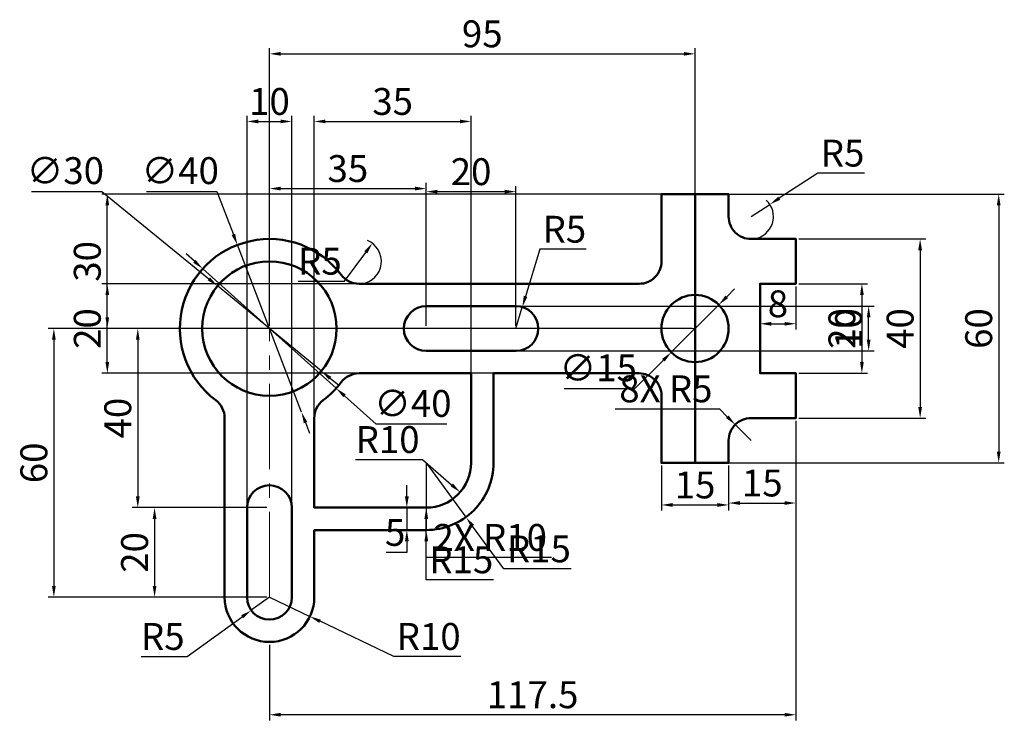
# Model space of a CAD drawing. Units: millimetres. Extents: x 35 to 255, y -2 to 154.
import ezdxf

# ---------------------------------------------------------------- set-up
doc = ezdxf.new("R2010")
doc.units = ezdxf.units.MM
doc.linetypes.add('CENTER2', pattern=[28.575, 19.05, -3.175, 3.175, -3.175])
for name, color, linetype, lineweight in [('M-CNTR', 4, 'CENTER2', 18), ('M-DIMS', 2, 'Continuous', 25), ('M-OUTL', 7, 'Continuous', 50)]:
    doc.layers.add(name, color=color, linetype=linetype, lineweight=lineweight)
doc.styles.get("Standard").update_dxf_attribs({"font": 'arial.ttf'})
doc.dimstyles.new('ISO-25', dxfattribs={"dimtxt": 6, "dimasz": 2.5, "dimexe": 1.25, "dimexo": 0.625, "dimtad": 1, "dimtoh": 1, "dimdec": 0, "dimtxsty": 'Standard', "dimcen": 2.5, "dimadec": 0, "dimazin": 0, "dimtfac": 1, "dimtdec": 0, "dimtmove": 0, "dimatfit": 3, "dimfxl": 1, "dimarcsym": 0})

# ---------------------------------------------------------------- blocks, each defined once
blk = doc.blocks.new('*D1')
at = {"layer": 'Defpoints', "color": 0, "transparency": 16777216}
for p in [(186.1, 146.8), (91.1, 85.45), (186.1, 85.45)]:
    blk.add_point(p, dxfattribs=at)
at = {"layer": 'M-DIMS', "color": 0, "lineweight": -2, "transparency": 16777216}
for p, q in [((91.1, 86.08), (91.1, 148.05)), ((186.1, 86.08), (186.1, 148.05)), ((93.6, 146.8), (183.6, 146.8))]:
    blk.add_line(p, q, dxfattribs=at)
at = {"layer": 'M-DIMS', "color": 0, "transparency": 16777216}
for points in [[(93.6, 147.22), (93.6, 146.39), (91.1, 146.8)], [(183.6, 147.22), (183.6, 146.39), (186.1, 146.8)]]:
    blk.add_solid(points, dxfattribs=at)
at = {"layer": 'M-DIMS', "color": 0, "transparency": 16777216, "insert": (138.6, 150.49), "char_height": 6, "attachment_point": 5}
blk.add_mtext('95', dxfattribs=at)
blk = doc.blocks.new('*D2')
at = {"layer": 'Defpoints', "color": 0, "transparency": 16777216}
for p in [(126.1, 116.71), (91.1, 85.45), (126.1, 85.45)]:
    blk.add_point(p, dxfattribs=at)
at = {"layer": 'M-DIMS', "color": 0, "lineweight": -2, "transparency": 16777216}
for p, q in [((91.1, 86.08), (91.1, 117.96)), ((93.6, 116.71), (123.6, 116.71)), ((126.1, 86.08), (126.1, 117.96))]:
    blk.add_line(p, q, dxfattribs=at)
at = {"layer": 'M-DIMS', "color": 0, "transparency": 16777216}
for points in [[(93.6, 117.13), (93.6, 116.3), (91.1, 116.71)], [(123.6, 117.13), (123.6, 116.3), (126.1, 116.71)]]:
    blk.add_solid(points, dxfattribs=at)
at = {"layer": 'M-DIMS', "color": 0, "transparency": 16777216, "insert": (108.6, 120.4), "char_height": 6, "attachment_point": 5}
blk.add_mtext('35', dxfattribs=at)
blk = doc.blocks.new('*D3')
at = {"layer": 'Defpoints', "color": 0, "transparency": 16777216}
for p in [(146.1, 116.02), (126.1, 85.45), (146.1, 85.45)]:
    blk.add_point(p, dxfattribs=at)
at = {"layer": 'M-DIMS', "color": 0, "lineweight": -2, "transparency": 16777216}
for p, q in [((126.1, 86.08), (126.1, 117.27)), ((146.1, 86.08), (146.1, 117.27)), ((128.6, 116.02), (143.6, 116.02))]:
    blk.add_line(p, q, dxfattribs=at)
at = {"layer": 'M-DIMS', "color": 0, "transparency": 16777216}
for points in [[(128.6, 116.44), (128.6, 115.61), (126.1, 116.02)], [(143.6, 116.44), (143.6, 115.61), (146.1, 116.02)]]:
    blk.add_solid(points, dxfattribs=at)
at = {"layer": 'M-DIMS', "color": 0, "transparency": 16777216, "insert": (136.1, 119.71), "char_height": 6, "attachment_point": 5}
blk.add_mtext('20', dxfattribs=at)
blk = doc.blocks.new('*D4')
at = {"layer": 'Defpoints', "color": 0, "transparency": 16777216}
for p in [(202.79, 113.18), (198.6, 110.45)]:
    blk.add_point(p, dxfattribs=at)
at = {"layer": 'M-DIMS', "color": 0, "lineweight": -2, "transparency": 16777216}
for p, q in [((213.54, 120.17), (204.89, 114.54)), ((223.89, 120.17), (213.54, 120.17)), ((198.6, 110.45), (202.79, 113.18))]:
    blk.add_line(p, q, dxfattribs=at)
blk.add_arc((198.6, 110.45), 5, 277.162, 47.3684, dxfattribs=at)
at = {"layer": 'M-DIMS', "color": 0, "transparency": 16777216}
blk.add_solid([(204.66, 114.89), (205.12, 114.19), (202.79, 113.18)], dxfattribs=at)
at = {"layer": 'M-DIMS', "color": 0, "transparency": 16777216, "insert": (219.03, 123.85), "char_height": 6, "attachment_point": 5}
blk.add_mtext('R5', dxfattribs=at)
blk = doc.blocks.new('*D5')
at = {"layer": 'Defpoints', "color": 0, "transparency": 16777216}
for p in [(200.6, 95.45), (208.6, 95.45), (208.6, 86.52)]:
    blk.add_point(p, dxfattribs=at)
at = {"layer": 'M-DIMS', "color": 0, "lineweight": -2, "transparency": 16777216}
for p, q in [((200.6, 94.83), (200.6, 85.27)), ((208.6, 94.83), (208.6, 85.27)), ((203.1, 86.52), (206.1, 86.52))]:
    blk.add_line(p, q, dxfattribs=at)
at = {"layer": 'M-DIMS', "color": 0, "transparency": 16777216}
for points in [[(203.1, 86.93), (203.1, 86.1), (200.6, 86.52)], [(206.1, 86.93), (206.1, 86.1), (208.6, 86.52)]]:
    blk.add_solid(points, dxfattribs=at)
at = {"layer": 'M-DIMS', "color": 0, "transparency": 16777216, "insert": (204.6, 90.2), "char_height": 6, "attachment_point": 5}
blk.add_mtext('8', dxfattribs=at)
blk = doc.blocks.new('*D6')
at = {"layer": 'Defpoints', "color": 0, "transparency": 16777216}
for p in [(208.6, 95.45), (208.6, 75.45), (223.34, 75.45)]:
    blk.add_point(p, dxfattribs=at)
at = {"layer": 'M-DIMS', "color": 0, "lineweight": -2, "transparency": 16777216}
for p, q in [((209.23, 95.45), (224.59, 95.45)), ((223.34, 92.95), (223.34, 77.95)), ((209.23, 75.45), (224.59, 75.45))]:
    blk.add_line(p, q, dxfattribs=at)
at = {"layer": 'M-DIMS', "color": 0, "transparency": 16777216}
for points in [[(222.93, 92.95), (223.76, 92.95), (223.34, 95.45)], [(222.93, 77.95), (223.76, 77.95), (223.34, 75.45)]]:
    blk.add_solid(points, dxfattribs=at)
at = {"layer": 'M-DIMS', "color": 0, "transparency": 16777216, "insert": (219.66, 85.45), "char_height": 6, "attachment_point": 5, "rotation": 90}
blk.add_mtext('20', dxfattribs=at)
blk = doc.blocks.new('*D7')
at = {"layer": 'Defpoints', "color": 0, "transparency": 16777216}
for p in [(208.6, 105.45), (208.6, 65.45), (236.34, 65.45)]:
    blk.add_point(p, dxfattribs=at)
at = {"layer": 'M-DIMS', "color": 0, "lineweight": -2, "transparency": 16777216}
for p, q in [((209.23, 105.45), (237.59, 105.45)), ((236.34, 102.95), (236.34, 67.95)), ((209.23, 65.45), (237.59, 65.45))]:
    blk.add_line(p, q, dxfattribs=at)
at = {"layer": 'M-DIMS', "color": 0, "transparency": 16777216}
for points in [[(235.92, 102.95), (236.76, 102.95), (236.34, 105.45)], [(235.92, 67.95), (236.76, 67.95), (236.34, 65.45)]]:
    blk.add_solid(points, dxfattribs=at)
at = {"layer": 'M-DIMS', "color": 0, "transparency": 16777216, "insert": (232.65, 85.45), "char_height": 6, "attachment_point": 5, "rotation": 90}
blk.add_mtext('40', dxfattribs=at)
blk = doc.blocks.new('*D8')
at = {"layer": 'Defpoints', "color": 0, "transparency": 16777216}
for p in [(178.6, 55.45), (193.6, 55.45), (193.6, 46.05)]:
    blk.add_point(p, dxfattribs=at)
at = {"layer": 'M-DIMS', "color": 0, "lineweight": -2, "transparency": 16777216}
for p, q in [((178.6, 54.83), (178.6, 44.8)), ((193.6, 54.83), (193.6, 44.8)), ((181.1, 46.05), (191.1, 46.05))]:
    blk.add_line(p, q, dxfattribs=at)
at = {"layer": 'M-DIMS', "color": 0, "transparency": 16777216}
for points in [[(181.1, 46.47), (181.1, 45.63), (178.6, 46.05)], [(191.1, 46.47), (191.1, 45.63), (193.6, 46.05)]]:
    blk.add_solid(points, dxfattribs=at)
at = {"layer": 'M-DIMS', "color": 0, "transparency": 16777216, "insert": (186.1, 49.74), "char_height": 6, "attachment_point": 5}
blk.add_mtext('15', dxfattribs=at)
blk = doc.blocks.new('*D9')
at = {"layer": 'Defpoints', "color": 0, "transparency": 16777216}
for p in [(208.6, 65.45), (193.6, 55.45), (208.6, 46.48)]:
    blk.add_point(p, dxfattribs=at)
at = {"layer": 'M-DIMS', "color": 0, "lineweight": -2, "transparency": 16777216}
for p, q in [((208.6, 64.83), (208.6, 45.23)), ((193.6, 54.83), (193.6, 45.23)), ((196.1, 46.48), (206.1, 46.48))]:
    blk.add_line(p, q, dxfattribs=at)
at = {"layer": 'M-DIMS', "color": 0, "transparency": 16777216}
for points in [[(196.1, 46.9), (196.1, 46.07), (193.6, 46.48)], [(206.1, 46.9), (206.1, 46.07), (208.6, 46.48)]]:
    blk.add_solid(points, dxfattribs=at)
at = {"layer": 'M-DIMS', "color": 0, "transparency": 16777216, "insert": (201.1, 50.17), "char_height": 6, "attachment_point": 5}
blk.add_mtext('15', dxfattribs=at)
blk = doc.blocks.new('*D10')
at = {"layer": 'Defpoints', "color": 0, "transparency": 16777216}
for p in [(186.1, 115.45), (186.1, 55.45), (253.88, 55.45)]:
    blk.add_point(p, dxfattribs=at)
at = {"layer": 'M-DIMS', "color": 0, "lineweight": -2, "transparency": 16777216}
for p, q in [((186.73, 115.45), (255.13, 115.45)), ((253.88, 112.95), (253.88, 57.95)), ((186.73, 55.45), (255.13, 55.45))]:
    blk.add_line(p, q, dxfattribs=at)
at = {"layer": 'M-DIMS', "color": 0, "transparency": 16777216}
for points in [[(253.46, 112.95), (254.3, 112.95), (253.88, 115.45)], [(253.46, 57.95), (254.3, 57.95), (253.88, 55.45)]]:
    blk.add_solid(points, dxfattribs=at)
at = {"layer": 'M-DIMS', "color": 0, "transparency": 16777216, "insert": (250.19, 85.45), "char_height": 6, "attachment_point": 5, "rotation": 90}
blk.add_mtext('60', dxfattribs=at)
blk = doc.blocks.new('*D11')
at = {"layer": 'Defpoints', "color": 0, "transparency": 16777216}
for p in [(147.54, 90.24), (146.1, 85.45)]:
    blk.add_point(p, dxfattribs=at)
at = {"layer": 'M-DIMS', "color": 0, "lineweight": -2, "transparency": 16777216}
for p, q in [((151.44, 103.18), (148.27, 92.64)), ((161.79, 103.18), (151.44, 103.18)), ((146.1, 85.45), (147.54, 90.24))]:
    blk.add_line(p, q, dxfattribs=at)
at = {"layer": 'M-DIMS', "color": 0, "transparency": 16777216}
blk.add_solid([(147.87, 92.76), (148.66, 92.51), (147.54, 90.24)], dxfattribs=at)
at = {"layer": 'M-DIMS', "color": 0, "transparency": 16777216, "insert": (156.93, 106.85), "char_height": 6, "attachment_point": 5}
blk.add_mtext('R5', dxfattribs=at)
blk = doc.blocks.new('*D12')
at = {"layer": 'Defpoints', "color": 0, "transparency": 16777216}
for p in [(114.07, 104.48), (111.1, 100.45)]:
    blk.add_point(p, dxfattribs=at)
at = {"layer": 'M-DIMS', "color": 0, "lineweight": -2, "transparency": 16777216}
for p, q in [((107.85, 96.04), (112.58, 102.47)), ((97.5, 96.04), (107.85, 96.04))]:
    blk.add_line(p, q, dxfattribs=at)
blk.add_arc((111.1, 100.45), 5, 277.162, 67.9535, dxfattribs=at)
at = {"layer": 'M-DIMS', "color": 0, "transparency": 16777216}
blk.add_solid([(112.25, 102.71), (112.92, 102.22), (114.07, 104.48)], dxfattribs=at)
at = {"layer": 'M-DIMS', "color": 0, "transparency": 16777216, "insert": (102.36, 99.71), "char_height": 6, "attachment_point": 5}
blk.add_mtext('R5', dxfattribs=at)
blk = doc.blocks.new('*D13')
at = {"layer": 'Defpoints', "color": 0, "transparency": 16777216}
for p in [(126.1, 55.45), (133.66, 48.91)]:
    blk.add_point(p, dxfattribs=at)
at = {"layer": 'M-DIMS', "color": 0, "lineweight": -2, "transparency": 16777216}
for p, q in [((110.31, 56.19), (125.25, 56.19)), ((125.25, 56.19), (131.77, 50.55))]:
    blk.add_line(p, q, dxfattribs=at)
at = {"layer": 'M-DIMS', "color": 0, "transparency": 16777216}
blk.add_solid([(132.05, 50.86), (131.5, 50.23), (133.66, 48.91)], dxfattribs=at)
at = {"layer": 'M-DIMS', "color": 0, "transparency": 16777216, "insert": (117.47, 59.88), "char_height": 6, "attachment_point": 5}
blk.add_mtext('R10', dxfattribs=at)
blk = doc.blocks.new('*D14')
at = {"layer": 'Defpoints', "color": 0, "transparency": 16777216}
for p in [(126.1, 55.45), (134.96, 43.35)]:
    blk.add_point(p, dxfattribs=at)
at = {"layer": 'M-DIMS', "color": 0, "lineweight": -2, "transparency": 16777216}
for p, q in [((126.1, 55.45), (134.96, 43.35)), ((143.43, 31.77), (136.43, 41.33)), ((158.44, 31.77), (143.43, 31.77))]:
    blk.add_line(p, q, dxfattribs=at)
at = {"layer": 'M-DIMS', "color": 0, "transparency": 16777216}
blk.add_solid([(136.77, 41.58), (136.1, 41.08), (134.96, 43.35)], dxfattribs=at)
at = {"layer": 'M-DIMS', "color": 0, "transparency": 16777216, "insert": (151.24, 35.46), "char_height": 6, "attachment_point": 5}
blk.add_mtext('R15', dxfattribs=at)
blk = doc.blocks.new('*D15')
at = {"layer": 'Defpoints', "color": 0, "transparency": 16777216}
for p in [(119.82, 45.45), (119.82, 40.45), (121.77, 40.45)]:
    blk.add_point(p, dxfattribs=at)
at = {"layer": 'M-DIMS', "color": 0, "lineweight": -2, "transparency": 16777216}
for p, q in [((121.77, 47.95), (121.77, 50.45)), ((120.45, 45.45), (123.02, 45.45)), ((121.77, 45.45), (121.77, 40.45)), ((120.45, 40.45), (123.02, 40.45)), ((121.77, 37.95), (121.77, 35.45)), ((121.77, 35.45), (117.17, 35.45))]:
    blk.add_line(p, q, dxfattribs=at)
at = {"layer": 'M-DIMS', "color": 0, "transparency": 16777216}
for points in [[(121.35, 47.95), (122.19, 47.95), (121.77, 45.45)], [(121.35, 37.95), (122.19, 37.95), (121.77, 40.45)]]:
    blk.add_solid(points, dxfattribs=at)
at = {"layer": 'M-DIMS', "color": 0, "transparency": 16777216, "insert": (119.16, 39.13), "char_height": 6, "attachment_point": 5}
blk.add_mtext('5', dxfattribs=at)
blk = doc.blocks.new('*D16')
at = {"layer": 'Defpoints', "color": 0, "transparency": 16777216}
for p in [(91.1, 45.45), (65.46, 25.45), (91.1, 25.45)]:
    blk.add_point(p, dxfattribs=at)
at = {"layer": 'M-DIMS', "color": 0, "lineweight": -2, "transparency": 16777216}
for p, q in [((90.48, 45.45), (64.21, 45.45)), ((65.46, 42.95), (65.46, 27.95)), ((90.48, 25.45), (64.21, 25.45))]:
    blk.add_line(p, q, dxfattribs=at)
at = {"layer": 'M-DIMS', "color": 0, "transparency": 16777216}
for points in [[(65.04, 42.95), (65.87, 42.95), (65.46, 45.45)], [(65.04, 27.95), (65.87, 27.95), (65.46, 25.45)]]:
    blk.add_solid(points, dxfattribs=at)
at = {"layer": 'M-DIMS', "color": 0, "transparency": 16777216, "insert": (61.77, 35.45), "char_height": 6, "attachment_point": 5, "rotation": 90}
blk.add_mtext('20', dxfattribs=at)
blk = doc.blocks.new('*D17')
at = {"layer": 'Defpoints', "color": 0, "transparency": 16777216}
for p in [(91.1, 85.45), (61.71, 45.45), (91.1, 45.45)]:
    blk.add_point(p, dxfattribs=at)
at = {"layer": 'M-DIMS', "color": 0, "lineweight": -2, "transparency": 16777216}
for p, q in [((90.48, 85.45), (60.46, 85.45)), ((61.71, 82.95), (61.71, 47.95)), ((90.48, 45.45), (60.46, 45.45))]:
    blk.add_line(p, q, dxfattribs=at)
at = {"layer": 'M-DIMS', "color": 0, "transparency": 16777216}
for points in [[(61.29, 82.95), (62.12, 82.95), (61.71, 85.45)], [(61.29, 47.95), (62.12, 47.95), (61.71, 45.45)]]:
    blk.add_solid(points, dxfattribs=at)
at = {"layer": 'M-DIMS', "color": 0, "transparency": 16777216, "insert": (58.02, 65.45), "char_height": 6, "attachment_point": 5, "rotation": 90}
blk.add_mtext('40', dxfattribs=at)
blk = doc.blocks.new('*D18')
at = {"layer": 'Defpoints', "color": 0, "transparency": 16777216}
for p in [(79.5, 94.96), (102.7, 75.95)]:
    blk.add_point(p, dxfattribs=at)
at = {"layer": 'M-DIMS', "color": 0, "lineweight": -2, "transparency": 16777216}
for p, q in [((37.99, 116.09), (53.72, 116.09)), ((53.72, 116.09), (77.57, 96.55)), ((102.7, 75.95), (79.5, 94.96)), ((104.64, 74.36), (106.57, 72.78))]:
    blk.add_line(p, q, dxfattribs=at)
at = {"layer": 'M-DIMS', "color": 0, "transparency": 16777216}
for points in [[(77.83, 96.87), (77.3, 96.22), (79.5, 94.96)], [(104.9, 74.68), (104.37, 74.04), (102.7, 75.95)]]:
    blk.add_solid(points, dxfattribs=at)
at = {"layer": 'M-DIMS', "color": 0, "transparency": 16777216, "insert": (45.54, 119.94), "char_height": 6, "attachment_point": 5}
blk.add_mtext('∅30', dxfattribs=at)
blk = doc.blocks.new('*D19')
at = {"layer": 'Defpoints', "color": 0, "transparency": 16777216}
for p in [(83.94, 104.13), (98.26, 66.78)]:
    blk.add_point(p, dxfattribs=at)
at = {"layer": 'M-DIMS', "color": 0, "lineweight": -2, "transparency": 16777216}
for p, q in [((63.63, 116.09), (79.36, 116.09)), ((79.36, 116.09), (83.05, 106.46)), ((98.26, 66.78), (83.94, 104.13)), ((99.16, 64.45), (100.05, 62.11))]:
    blk.add_line(p, q, dxfattribs=at)
at = {"layer": 'M-DIMS', "color": 0, "transparency": 16777216}
for points in [[(83.44, 106.61), (82.66, 106.31), (83.94, 104.13)], [(99.55, 64.59), (98.77, 64.3), (98.26, 66.78)]]:
    blk.add_solid(points, dxfattribs=at)
at = {"layer": 'M-DIMS', "color": 0, "transparency": 16777216, "insert": (71.18, 119.94), "char_height": 6, "attachment_point": 5}
blk.add_mtext('∅40', dxfattribs=at)
blk = doc.blocks.new('*D20')
at = {"layer": 'Defpoints', "color": 0, "transparency": 16777216}
for p in [(91.1, 25.45), (100.13, 21.15)]:
    blk.add_point(p, dxfattribs=at)
at = {"layer": 'M-DIMS', "color": 0, "lineweight": -2, "transparency": 16777216}
for p, q in [((91.1, 25.45), (100.13, 21.15)), ((118.86, 12.22), (102.39, 20.07)), ((133.8, 12.22), (118.86, 12.22))]:
    blk.add_line(p, q, dxfattribs=at)
at = {"layer": 'M-DIMS', "color": 0, "transparency": 16777216}
blk.add_solid([(102.56, 20.45), (102.21, 19.7), (100.13, 21.15)], dxfattribs=at)
at = {"layer": 'M-DIMS', "color": 0, "transparency": 16777216, "insert": (126.64, 15.91), "char_height": 6, "attachment_point": 5}
blk.add_mtext('R10', dxfattribs=at)
blk = doc.blocks.new('*D21')
at = {"layer": 'Defpoints', "color": 0, "transparency": 16777216}
for p in [(91.1, 25.45), (87.05, 22.53)]:
    blk.add_point(p, dxfattribs=at)
at = {"layer": 'M-DIMS', "color": 0, "lineweight": -2, "transparency": 16777216}
for p, q in [((91.1, 25.45), (87.05, 22.53)), ((72.77, 12.22), (85.02, 21.06)), ((62.43, 12.22), (72.77, 12.22))]:
    blk.add_line(p, q, dxfattribs=at)
at = {"layer": 'M-DIMS', "color": 0, "transparency": 16777216}
blk.add_solid([(84.78, 21.4), (85.27, 20.73), (87.05, 22.53)], dxfattribs=at)
at = {"layer": 'M-DIMS', "color": 0, "transparency": 16777216, "insert": (67.29, 15.9), "char_height": 6, "attachment_point": 5}
blk.add_mtext('R5', dxfattribs=at)
blk = doc.blocks.new('*D22')
at = {"layer": 'Defpoints', "color": 0, "transparency": 16777216}
for p in [(91.1, 85.45), (42.98, 25.45), (91.1, 25.45)]:
    blk.add_point(p, dxfattribs=at)
at = {"layer": 'M-DIMS', "color": 0, "lineweight": -2, "transparency": 16777216}
for p, q in [((90.48, 85.45), (41.73, 85.45)), ((42.98, 82.95), (42.98, 27.95)), ((90.48, 25.45), (41.73, 25.45))]:
    blk.add_line(p, q, dxfattribs=at)
at = {"layer": 'M-DIMS', "color": 0, "transparency": 16777216}
for points in [[(42.56, 82.95), (43.39, 82.95), (42.98, 85.45)], [(42.56, 27.95), (43.39, 27.95), (42.98, 25.45)]]:
    blk.add_solid(points, dxfattribs=at)
at = {"layer": 'M-DIMS', "color": 0, "transparency": 16777216, "insert": (39.29, 55.45), "char_height": 6, "attachment_point": 5, "rotation": 90}
blk.add_mtext('60', dxfattribs=at)
blk = doc.blocks.new('SLOT-30X10')
blk.add_lwpolyline([(0, 5), (0, 25, -1), (10, 25), (10, 5, -1)], format="xyb", close=True)
blk = doc.blocks.new('*D24')
at = {"layer": 'Defpoints', "color": 0, "transparency": 16777216}
for p in [(208.6, 65.45), (91.1, 15.45), (91.1, -0.8)]:
    blk.add_point(p, dxfattribs=at)
at = {"layer": 'M-DIMS', "color": 0, "lineweight": -2, "transparency": 16777216}
for p, q in [((208.6, 64.83), (208.6, -2.05)), ((91.1, 14.83), (91.1, -2.05)), ((206.1, -0.8), (93.6, -0.8))]:
    blk.add_line(p, q, dxfattribs=at)
at = {"layer": 'M-DIMS', "color": 0, "transparency": 16777216}
for points in [[(93.6, -0.38), (93.6, -1.21), (91.1, -0.8)], [(206.1, -0.38), (206.1, -1.21), (208.6, -0.8)]]:
    blk.add_solid(points, dxfattribs=at)
at = {"layer": 'M-DIMS', "color": 0, "transparency": 16777216, "insert": (149.85, 2.89), "char_height": 6, "attachment_point": 5}
blk.add_mtext('117.5', dxfattribs=at)
blk = doc.blocks.new('*D25')
at = {"layer": 'Defpoints', "color": 0, "transparency": 16777216}
for p in [(54.91, 115.45), (186.1, 115.45), (186.1, 85.45)]:
    blk.add_point(p, dxfattribs=at)
at = {"layer": 'M-DIMS', "color": 0, "lineweight": -2, "transparency": 16777216}
for p, q in [((185.48, 115.45), (53.66, 115.45)), ((54.91, 87.95), (54.91, 112.95)), ((185.48, 85.45), (53.66, 85.45))]:
    blk.add_line(p, q, dxfattribs=at)
at = {"layer": 'M-DIMS', "color": 0, "transparency": 16777216}
for points in [[(54.49, 112.95), (55.32, 112.95), (54.91, 115.45)], [(54.49, 87.95), (55.32, 87.95), (54.91, 85.45)]]:
    blk.add_solid(points, dxfattribs=at)
at = {"layer": 'M-DIMS', "color": 0, "transparency": 16777216, "insert": (51.21, 100.45), "char_height": 6, "attachment_point": 5, "rotation": 90}
blk.add_mtext('30', dxfattribs=at)
blk = doc.blocks.new('*D26')
at = {"layer": 'Defpoints', "color": 0, "transparency": 16777216}
for p in [(96.1, 131.7), (86.1, 45.45), (96.1, 45.45)]:
    blk.add_point(p, dxfattribs=at)
at = {"layer": 'M-DIMS', "color": 0, "lineweight": -2, "transparency": 16777216}
for p, q in [((86.1, 46.08), (86.1, 132.95)), ((96.1, 46.08), (96.1, 132.95)), ((88.6, 131.7), (93.6, 131.7))]:
    blk.add_line(p, q, dxfattribs=at)
at = {"layer": 'M-DIMS', "color": 0, "transparency": 16777216}
for points in [[(88.6, 132.12), (88.6, 131.29), (86.1, 131.7)], [(93.6, 132.12), (93.6, 131.29), (96.1, 131.7)]]:
    blk.add_solid(points, dxfattribs=at)
at = {"layer": 'M-DIMS', "color": 0, "transparency": 16777216, "insert": (91.1, 135.39), "char_height": 6, "attachment_point": 5}
blk.add_mtext('10', dxfattribs=at)
blk = doc.blocks.new('*D27')
at = {"layer": 'Defpoints', "color": 0, "transparency": 16777216}
for p in [(146.1, 90.45), (224.85, 90.45), (146.1, 80.45)]:
    blk.add_point(p, dxfattribs=at)
at = {"layer": 'M-DIMS', "color": 0, "lineweight": -2, "transparency": 16777216}
for p, q in [((146.73, 90.45), (226.1, 90.45)), ((224.85, 82.95), (224.85, 87.95)), ((146.73, 80.45), (226.1, 80.45))]:
    blk.add_line(p, q, dxfattribs=at)
at = {"layer": 'M-DIMS', "color": 0, "transparency": 16777216}
for points in [[(224.44, 87.95), (225.27, 87.95), (224.85, 90.45)], [(224.44, 82.95), (225.27, 82.95), (224.85, 80.45)]]:
    blk.add_solid(points, dxfattribs=at)
at = {"layer": 'M-DIMS', "color": 0, "transparency": 16777216, "insert": (221.16, 85.45), "char_height": 6, "attachment_point": 5, "rotation": 90}
blk.add_mtext('10', dxfattribs=at)
blk = doc.blocks.new('*D28')
at = {"layer": 'Defpoints', "color": 0, "transparency": 16777216}
for p in [(136.1, 131.7), (136.1, 55.45), (101.1, 45.45)]:
    blk.add_point(p, dxfattribs=at)
at = {"layer": 'M-DIMS', "color": 0, "lineweight": -2, "transparency": 16777216}
for p, q in [((101.1, 46.08), (101.1, 132.95)), ((136.1, 56.08), (136.1, 132.95)), ((103.6, 131.7), (133.6, 131.7))]:
    blk.add_line(p, q, dxfattribs=at)
at = {"layer": 'M-DIMS', "color": 0, "transparency": 16777216}
for points in [[(103.6, 132.12), (103.6, 131.29), (101.1, 131.7)], [(133.6, 132.12), (133.6, 131.29), (136.1, 131.7)]]:
    blk.add_solid(points, dxfattribs=at)
at = {"layer": 'M-DIMS', "color": 0, "transparency": 16777216, "insert": (118.6, 135.39), "char_height": 6, "attachment_point": 5}
blk.add_mtext('35', dxfattribs=at)
blk = doc.blocks.new('*D29')
at = {"layer": 'Defpoints', "color": 0, "transparency": 16777216}
for p in [(54.91, 95.45), (173.6, 95.45), (173.6, 75.45)]:
    blk.add_point(p, dxfattribs=at)
at = {"layer": 'M-DIMS', "color": 0, "lineweight": -2, "transparency": 16777216}
for p, q in [((172.98, 95.45), (53.66, 95.45)), ((54.91, 77.95), (54.91, 92.95)), ((172.98, 75.45), (53.66, 75.45))]:
    blk.add_line(p, q, dxfattribs=at)
at = {"layer": 'M-DIMS', "color": 0, "transparency": 16777216}
for points in [[(54.49, 92.95), (55.32, 92.95), (54.91, 95.45)], [(54.49, 77.95), (55.32, 77.95), (54.91, 75.45)]]:
    blk.add_solid(points, dxfattribs=at)
at = {"layer": 'M-DIMS', "color": 0, "transparency": 16777216, "insert": (51.22, 85.45), "char_height": 6, "attachment_point": 5, "rotation": 90}
blk.add_mtext('20', dxfattribs=at)
blk = doc.blocks.new('*D30')
at = {"layer": 'Defpoints', "color": 0, "transparency": 16777216}
for p in [(76.21, 98.8), (105.99, 72.1)]:
    blk.add_point(p, dxfattribs=at)
at = {"layer": 'M-DIMS', "color": 0, "lineweight": -2, "transparency": 16777216}
for p, q in [((74.35, 100.47), (72.49, 102.14)), ((76.21, 98.8), (105.99, 72.1)), ((114.93, 64.1), (107.86, 70.44)), ((130.66, 64.1), (114.93, 64.1))]:
    blk.add_line(p, q, dxfattribs=at)
at = {"layer": 'M-DIMS', "color": 0, "transparency": 16777216}
for points in [[(74.63, 100.78), (74.07, 100.16), (76.21, 98.8)], [(108.13, 70.75), (107.58, 70.13), (105.99, 72.1)]]:
    blk.add_solid(points, dxfattribs=at)
at = {"layer": 'M-DIMS', "color": 0, "transparency": 16777216, "insert": (123.11, 67.95), "char_height": 6, "attachment_point": 5}
blk.add_mtext('∅40', dxfattribs=at)
blk = doc.blocks.new('*D31')
at = {"layer": 'Defpoints', "color": 0, "transparency": 16777216}
for p in [(191.4, 90.76), (180.8, 80.15)]:
    blk.add_point(p, dxfattribs=at)
at = {"layer": 'M-DIMS', "color": 0, "lineweight": -2, "transparency": 16777216}
for p, q in [((193.17, 92.53), (194.94, 94.29)), ((191.4, 90.76), (180.8, 80.15)), ((172.69, 72.04), (179.03, 78.38)), ((156.9, 72.04), (172.69, 72.04))]:
    blk.add_line(p, q, dxfattribs=at)
at = {"layer": 'M-DIMS', "color": 0, "transparency": 16777216}
for points in [[(192.88, 92.82), (193.47, 92.23), (191.4, 90.76)], [(178.74, 78.68), (179.33, 78.09), (180.8, 80.15)]]:
    blk.add_solid(points, dxfattribs=at)
at = {"layer": 'M-DIMS', "color": 0, "transparency": 16777216, "insert": (164.49, 75.9), "char_height": 6, "attachment_point": 5}
blk.add_mtext('∅15', dxfattribs=at)
blk = doc.blocks.new('*D32')
at = {"layer": 'Defpoints', "color": 0, "transparency": 16777216}
for p in [(126.1, 55.45), (126.1, 40.45)]:
    blk.add_point(p, dxfattribs=at)
at = {"layer": 'M-DIMS', "color": 0, "lineweight": -2, "transparency": 16777216}
for p, q in [((126.1, 55.45), (126.1, 40.45)), ((126.1, 29.33), (126.1, 37.95)), ((141.11, 29.33), (126.1, 29.33))]:
    blk.add_line(p, q, dxfattribs=at)
at = {"layer": 'M-DIMS', "color": 0, "transparency": 16777216}
blk.add_solid([(126.52, 37.95), (125.69, 37.95), (126.1, 40.45)], dxfattribs=at)
at = {"layer": 'M-DIMS', "color": 0, "transparency": 16777216, "insert": (133.92, 33.02), "char_height": 6, "attachment_point": 5}
blk.add_mtext('R15', dxfattribs=at)
blk = doc.blocks.new('*D33')
at = {"layer": 'Defpoints', "color": 0, "transparency": 16777216}
for p in [(126.1, 55.45), (126.1, 45.45)]:
    blk.add_point(p, dxfattribs=at)
at = {"layer": 'M-DIMS', "color": 0, "lineweight": -2, "transparency": 16777216}
for p, q in [((126.1, 55.45), (126.1, 45.45)), ((126.1, 34.33), (126.1, 42.95)), ((154.04, 34.33), (126.1, 34.33))]:
    blk.add_line(p, q, dxfattribs=at)
at = {"layer": 'M-DIMS', "color": 0, "transparency": 16777216}
blk.add_solid([(126.52, 42.95), (125.69, 42.95), (126.1, 45.45)], dxfattribs=at)
at = {"layer": 'M-DIMS', "color": 0, "transparency": 16777216, "insert": (140.38, 38.02), "char_height": 6, "attachment_point": 5}
blk.add_mtext('2X R10', dxfattribs=at)
blk = doc.blocks.new('*D34')
at = {"layer": 'Defpoints', "color": 0, "transparency": 16777216}
for p in [(195.07, 63.99), (198.6, 60.45)]:
    blk.add_point(p, dxfattribs=at)
at = {"layer": 'M-DIMS', "color": 0, "lineweight": -2, "transparency": 16777216}
for p, q in [((168.28, 67.52), (191.53, 67.52)), ((191.53, 67.52), (193.3, 65.76)), ((198.6, 60.45), (195.07, 63.99))]:
    blk.add_line(p, q, dxfattribs=at)
at = {"layer": 'M-DIMS', "color": 0, "transparency": 16777216}
blk.add_solid([(193.59, 66.05), (193, 65.46), (195.07, 63.99)], dxfattribs=at)
at = {"layer": 'M-DIMS', "color": 0, "transparency": 16777216, "insert": (179.59, 71.21), "char_height": 6, "attachment_point": 5}
blk.add_mtext('8X R5', dxfattribs=at)

msp = doc.modelspace()

# ---------------------------------------------------------------- linework, layer by layer
at = {"layer": 'M-CNTR'}
msp.add_lwpolyline([(91.1, 25.45), (91.1, 85.45), (186.1, 85.45)], dxfattribs=at)
at = {"layer": 'M-OUTL'}
for points in [[(186.1, 115.45), (178.6, 115.45), (178.6, 100.45, -0.414214), (173.6, 95.45), (111.1, 95.45, -0.236068), (107.1, 97.45, 1.15301), (79.1, 69.45, -0.236068), (81.1, 65.45), (81.1, 25.45, 1), (101.1, 25.45)], [(101.1, 25.45), (101.1, 40.45), (126.1, 40.45, 0.414214), (141.1, 55.45), (141.1, 75.45), (173.6, 75.45, -0.414214), (178.6, 70.45), (178.6, 55.45), (186.1, 55.45)]]:
    msp.add_lwpolyline(points, format="xyb", dxfattribs=at)
for points in [[(193.6, 110.45, 0.414214), (198.6, 105.45), (208.6, 105.45), (208.6, 95.45), (200.6, 95.45), (200.6, 75.45), (208.6, 75.45), (208.6, 65.45), (198.6, 65.45, 0.414214), (193.6, 60.45), (193.6, 55.45), (186.1, 55.45), (186.1, 85.45), (186.1, 115.45), (193.6, 115.45)], [(103.1, 69.45, 0.236068), (101.1, 65.45), (101.1, 45.45), (126.1, 45.45, 0.414214), (136.1, 55.45), (136.1, 75.45), (111.1, 75.45, 0.236068), (107.1, 73.45, -0.071068)]]:
    msp.add_lwpolyline(points, format="xyb", close=True, dxfattribs=at)
for centre, radius in [((91.1, 85.45), 15), ((186.1, 85.45), 7.5)]:
    msp.add_circle(centre, radius, dxfattribs=at)

# ---------------------------------------------------------------- block references
at = {"layer": 'M-OUTL', "extrusion": (0, 0, -1), "zscale": -1, "rotation": 90.00000000000006}
msp.add_blockref('SLOT-30X10', (-121.1, 80.45), dxfattribs=at)
at = {"layer": 'M-OUTL'}
msp.add_blockref('SLOT-30X10', (86.1, 20.45), dxfattribs=at)

# ---------------------------------------------------------------- dimensions: what is measured, and where the dimension line sits
at = {"layer": 'M-DIMS'}
for base, p1, p2, override, picture, middle in [((186.1, 146.8), (91.1, 85.45), (186.1, 85.45), {"dimclrd": 0, "dimclre": 0, "dimclrt": 0}, '*D1', (138.6, 150.49)), ((96.1, 131.7), (86.1, 45.45), (96.1, 45.45), {"dimdec": 0, "dimlfac": 1, "dimrnd": 0, "dimzin": 0, "dimdsep": 46, "dimlunit": 2}, '*D26', (91.1, 135.39)), ((136.1, 131.7), (101.1, 45.45), (136.1, 55.45), {"dimdec": 0, "dimlfac": 1, "dimrnd": 0, "dimzin": 0, "dimdsep": 46, "dimlunit": 2}, '*D28', (118.6, 135.39)), ((126.1, 116.71), (91.1, 85.45), (126.1, 85.45), {"dimclrd": 0, "dimclre": 0, "dimclrt": 0}, '*D2', (108.6, 120.4)), ((146.1, 116.02), (126.1, 85.45), (146.1, 85.45), {"dimclrd": 0, "dimclre": 0, "dimclrt": 0}, '*D3', (136.1, 119.71)), ((208.6, 86.52), (200.6, 95.45), (208.6, 95.45), {"dimclrd": 0, "dimclre": 0, "dimclrt": 0}, '*D5', (204.6, 90.2)), ((91.1, -0.8), (208.6, 65.45), (91.1, 15.45), {"dimdec": 1, "dimlfac": 1, "dimrnd": 0, "dimzin": 0, "dimdsep": 46, "dimlunit": 2}, '*D24', (149.85, 2.89)), ((208.6, 46.48), (193.6, 55.45), (208.6, 65.45), {"dimclrd": 0, "dimclre": 0, "dimclrt": 0}, '*D9', (201.1, 50.17)), ((193.6, 46.05), (178.6, 55.45), (193.6, 55.45), {"dimclrd": 0, "dimclre": 0, "dimclrt": 0}, '*D8', (186.1, 49.74))]:
    dim = msp.add_linear_dim(base=base, p1=p1, p2=p2, dimstyle='ISO-25', override=override, dxfattribs=at)
    dim.commit()
    dim.dimension.update_dxf_attribs({"geometry": picture, "text_midpoint": middle})
for center, mpoint, picture, middle in [((198.6, 110.45), (202.79, 113.18), '*D4', (219.03, 120.17)), ((146.1, 85.45), (147.54, 90.24), '*D11', (156.93, 103.18)), ((111.1, 100.45), (114.07, 104.48), '*D12', (102.36, 96.04)), ((126.1, 55.45), (133.66, 48.91), '*D13', (117.47, 56.19)), ((126.1, 55.45), (134.96, 43.35), '*D14', (151.24, 31.77)), ((91.1, 25.45), (87.05, 22.53), '*D21', (67.29, 12.22)), ((91.1, 25.45), (100.13, 21.15), '*D20', (126.64, 12.22))]:
    dim = msp.add_radius_dim(center=center, mpoint=mpoint, dimstyle='ISO-25', override={"dimclrd": 0, "dimclre": 0, "dimclrt": 0}, dxfattribs=at)
    dim.commit()
    dim.dimension.update_dxf_attribs({"geometry": picture, "text_midpoint": middle, "dimtype": 164})
for p1, p2, override, picture, middle in [((102.7, 75.95), (79.5, 94.96), {"dimclrd": 0, "dimclre": 0, "dimclrt": 0}, '*D18', (45.54, 116.09)), ((98.26, 66.78), (83.94, 104.13), {"dimclrd": 0, "dimclre": 0, "dimclrt": 0}, '*D19', (71.18, 116.09)), ((76.21, 98.8), (105.99, 72.1), {"dimdec": 0, "dimlfac": 1, "dimrnd": 0, "dimzin": 0, "dimdsep": 46, "dimlunit": 2}, '*D30', (123.11, 64.1))]:
    dim = msp.add_diameter_dim_2p(p1=p1, p2=p2, dimstyle='ISO-25', override=override, dxfattribs=at)
    dim.commit()
    dim.dimension.update_dxf_attribs({"geometry": picture, "text_midpoint": middle, "dimtype": 163})
for base, p1, p2, override, picture, middle in [((54.91, 115.45), (186.1, 85.45), (186.1, 115.45), {"dimdec": 0, "dimlfac": 1, "dimrnd": 0, "dimzin": 0, "dimdsep": 46, "dimlunit": 2}, '*D25', (51.21, 100.45)), ((253.88, 55.45), (186.1, 115.45), (186.1, 55.45), {"dimclrd": 0, "dimclre": 0, "dimclrt": 0}, '*D10', (250.19, 85.45)), ((236.34, 65.45), (208.6, 105.45), (208.6, 65.45), {"dimclrd": 0, "dimclre": 0, "dimclrt": 0}, '*D7', (232.65, 85.45)), ((54.91, 95.45), (173.6, 75.45), (173.6, 95.45), {"dimdec": 0, "dimlfac": 1, "dimrnd": 0, "dimzin": 0, "dimdsep": 46, "dimlunit": 2}, '*D29', (51.22, 85.45)), ((223.34, 75.45), (208.6, 95.45), (208.6, 75.45), {"dimclrd": 0, "dimclre": 0, "dimclrt": 0}, '*D6', (219.66, 85.45)), ((224.85, 90.45), (146.1, 80.45), (146.1, 90.45), {"dimdec": 0, "dimlfac": 1, "dimrnd": 0, "dimzin": 0, "dimdsep": 46, "dimlunit": 2}, '*D27', (221.16, 85.45)), ((42.98, 25.45), (91.1, 85.45), (91.1, 25.45), {"dimclrd": 0, "dimclre": 0, "dimclrt": 0}, '*D22', (39.29, 55.45)), ((61.71, 45.45), (91.1, 85.45), (91.1, 45.45), {"dimclrd": 0, "dimclre": 0, "dimclrt": 0}, '*D17', (58.02, 65.45)), ((121.77, 40.45), (119.82, 45.45), (119.82, 40.45), {"dimclrd": 0, "dimclre": 0, "dimclrt": 0}, '*D15', (119.16, 39.13)), ((65.46, 25.45), (91.1, 45.45), (91.1, 25.45), {"dimclrd": 0, "dimclre": 0, "dimclrt": 0}, '*D16', (61.77, 35.45))]:
    dim = msp.add_linear_dim(base=base, p1=p1, p2=p2, angle=90, dimstyle='ISO-25', override=override, dxfattribs=at)
    dim.commit()
    dim.dimension.update_dxf_attribs({"geometry": picture, "text_midpoint": middle})
dim = msp.add_diameter_dim_2p(p1=(191.4, 90.76), p2=(180.8, 80.15), dimstyle='ISO-25', override={"dimdec": 0, "dimlfac": 1, "dimrnd": 0, "dimzin": 0, "dimdsep": 46, "dimlunit": 2}, dxfattribs=at)
dim.commit()
dim.dimension.update_dxf_attribs({"geometry": '*D31', "text_midpoint": (164.49, 72.04)})
for center, mpoint, text, picture, middle in [((198.6, 60.45), (195.07, 63.99), '8X <>', '*D34', (179.59, 71.21)), ((126.1, 55.45), (126.1, 45.45), '2X <>', '*D33', (140.38, 38.02))]:
    dim = msp.add_radius_dim(center=center, mpoint=mpoint, text=text, dimstyle='ISO-25', override={"dimdec": 0, "dimlfac": 1, "dimrnd": 0, "dimzin": 0, "dimdsep": 46, "dimlunit": 2}, dxfattribs=at)
    dim.commit()
    dim.dimension.update_dxf_attribs({"geometry": picture, "text_midpoint": middle})
dim = msp.add_radius_dim(center=(126.1, 55.45), mpoint=(126.1, 40.45), dimstyle='ISO-25', override={"dimdec": 0, "dimlfac": 1, "dimrnd": 0, "dimzin": 0, "dimdsep": 46, "dimlunit": 2}, dxfattribs=at)
dim.commit()
dim.dimension.update_dxf_attribs({"geometry": '*D32', "text_midpoint": (133.92, 33.02)})

doc.saveas('drawing.dxf')
